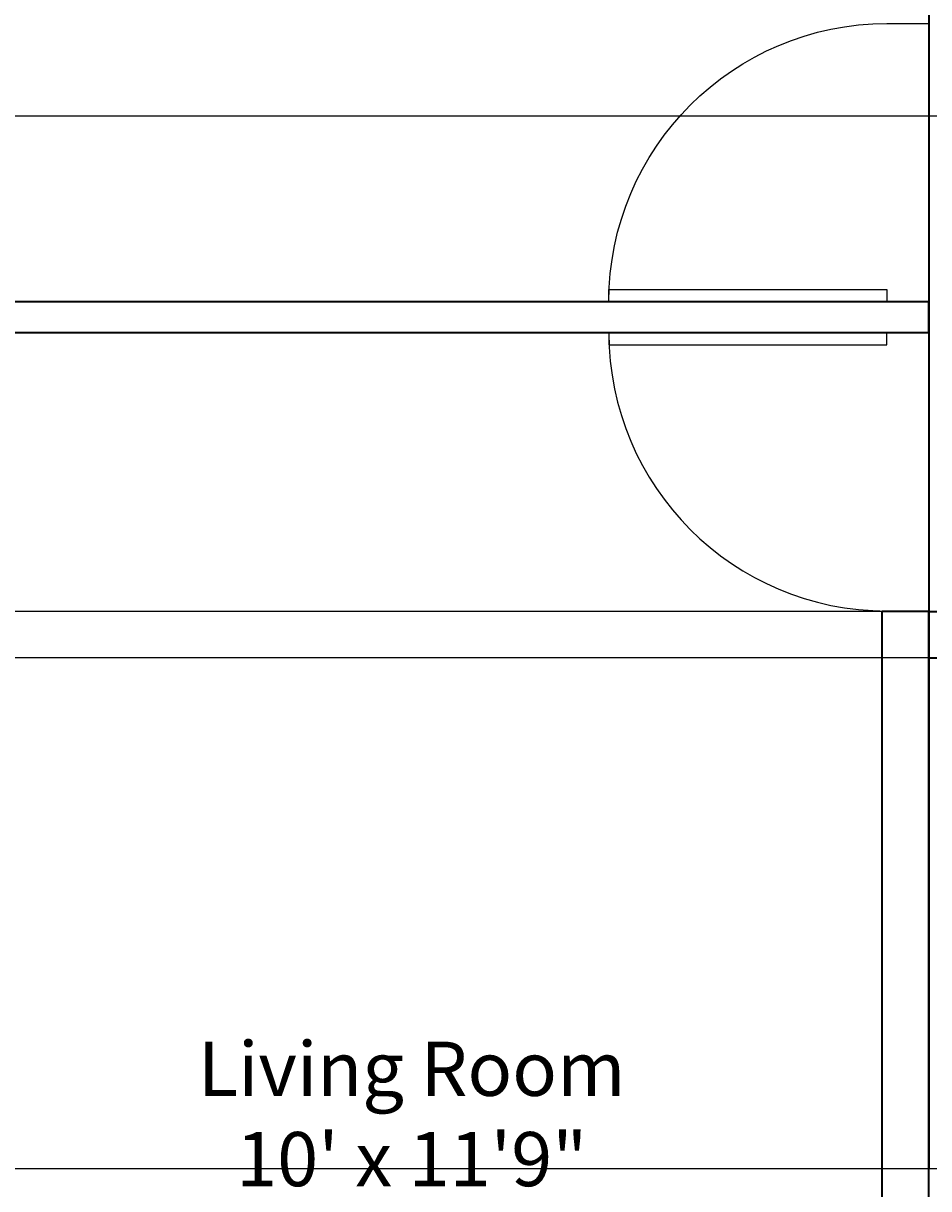
# Model space of a CAD drawing. Units: feet. Extents: x 105 to 1094, y -88 to 588.
# Tile 36 of 59: x 436 to 553, y 138 to 288. Entities that reach past the tile are written whole.
import ezdxf

# ---------------------------------------------------------------- set-up
doc = ezdxf.new("R2010")
doc.units = ezdxf.units.FT
doc.header["$MEASUREMENT"] = 0
for name, color, linetype, lineweight in [('A-ANNO-DIMS', 2, 'Continuous', 18), ('A-AREA-IDEN', 7, 'Continuous', 18), ('A-DOOR', 3, 'Continuous', 25), ('A-WALL', 7, 'Continuous', 35)]:
    doc.layers.add(name, color=color, linetype=linetype, lineweight=lineweight)
doc.styles.get("Standard").update_dxf_attribs({"font": 'arial.ttf'})
doc.dimstyles.get("Standard").update_dxf_attribs({"dimtxt": 0.18, "dimasz": 0.18, "dimexe": 0.18, "dimexo": 0.0625, "dimgap": 0.09, "dimtad": 0, "dimtih": 1, "dimtoh": 1, "dimdec": 4, "dimzin": 0, "dimdsep": 46, "dimtxsty": 'Standard', "dimcen": 0.09, "dimadec": 0, "dimazin": 0, "dimtfac": 1, "dimtdec": 4, "dimtofl": 0, "dimtmove": 0, "dimatfit": 3, "dimfxl": 1, "dimtolj": 1, "dimtzin": 0, "dimarcsym": 0})

# ---------------------------------------------------------------- blocks, each defined once
blk = doc.blocks.new('*U3')
for p, q in [((0, 0), (0, -6)), ((-40, 0), (-40, -6))]:
    blk.add_line(p, q)
blk.add_lwpolyline([(0, 0), (0, 40), (-1.75, 40), (-1.75, 0)], close=True)
blk.add_arc((0, 0), 40, 90, 180)
blk = doc.blocks.new('*D20')
at = {"layer": 'A-ANNO-DIMS', "color": 0, "lineweight": -2, "transparency": 16777216}
for p, q in [((150.69, 276.02), (150.69, -88.15)), ((1048.69, 276.02), (1048.69, -88.15)), ((150.87, -87.97), (599.4, -87.97)), ((1048.51, -87.97), (599.98, -87.97))]:
    blk.add_line(p, q, dxfattribs=at)
at = {"layer": 'A-ANNO-DIMS', "color": 0, "transparency": 16777216}
for points in [[(150.87, -87.94), (150.87, -88), (150.69, -87.97)], [(1048.51, -87.94), (1048.51, -88), (1048.69, -87.97)]]:
    blk.add_solid(points, dxfattribs=at)
at = {"layer": 'Defpoints', "color": 0, "transparency": 16777216}
for p in [(150.69, 276.08), (1048.69, 276.08), (1048.69, -87.97)]:
    blk.add_point(p, dxfattribs=at)
at = {"layer": 'A-ANNO-DIMS', "color": 0, "transparency": 16777216, "insert": (599.69, -87.97), "char_height": 0.18, "attachment_point": 5}
blk.add_mtext('\\A1;898', dxfattribs=at)
blk = doc.blocks.new('*D21')
at = {"layer": 'A-ANNO-DIMS', "color": 0, "lineweight": -2, "transparency": 16777216}
for p, q in [((849.63, 543.08), (105.46, 543.08)), ((105.64, 542.9), (105.64, 250.26)), ((105.64, -42.74), (105.64, 249.9)), ((849.63, -42.92), (105.46, -42.92))]:
    blk.add_line(p, q, dxfattribs=at)
at = {"layer": 'A-ANNO-DIMS', "color": 0, "transparency": 16777216}
for points in [[(105.61, 542.9), (105.67, 542.9), (105.64, 543.08)], [(105.61, -42.74), (105.67, -42.74), (105.64, -42.92)]]:
    blk.add_solid(points, dxfattribs=at)
at = {"layer": 'Defpoints', "color": 0, "transparency": 16777216}
for p in [(105.64, 543.08), (849.69, 543.08), (849.69, -42.92)]:
    blk.add_point(p, dxfattribs=at)
at = {"layer": 'A-ANNO-DIMS', "color": 0, "transparency": 16777216, "insert": (105.64, 250.08), "char_height": 0.18, "attachment_point": 5}
blk.add_mtext('\\A1;586', dxfattribs=at)
blk = doc.blocks.new('*D36')
at = {"layer": 'A-ANNO-DIMS', "color": 0, "lineweight": -2, "transparency": 16777216}
for p, q in [((547.24, 248.08), (105.46, 248.08)), ((105.64, 247.9), (105.64, 230.26)), ((105.64, 212.26), (105.64, 229.9)), ((546.63, 212.08), (105.46, 212.08))]:
    blk.add_line(p, q, dxfattribs=at)
at = {"layer": 'A-ANNO-DIMS', "color": 0, "transparency": 16777216}
for points in [[(105.61, 247.9), (105.67, 247.9), (105.64, 248.08)], [(105.61, 212.26), (105.67, 212.26), (105.64, 212.08)]]:
    blk.add_solid(points, dxfattribs=at)
at = {"layer": 'Defpoints', "color": 0, "transparency": 16777216}
for p in [(105.64, 248.08), (547.3, 248.08), (546.69, 212.08)]:
    blk.add_point(p, dxfattribs=at)
at = {"layer": 'A-ANNO-DIMS', "color": 0, "transparency": 16777216, "insert": (105.64, 230.08), "char_height": 0.18, "attachment_point": 5}
blk.add_mtext('\\A1;36', dxfattribs=at)
blk = doc.blocks.new('*D46')
at = {"layer": 'A-ANNO-DIMS', "color": 0, "lineweight": -2, "transparency": 16777216}
for p, q in [((580.63, 206.08), (105.46, 206.08)), ((105.64, 205.9), (105.64, 173.26)), ((105.64, 140.26), (105.64, 172.9)), ((580.63, 140.08), (105.46, 140.08))]:
    blk.add_line(p, q, dxfattribs=at)
at = {"layer": 'A-ANNO-DIMS', "color": 0, "transparency": 16777216}
for points in [[(105.61, 205.9), (105.67, 205.9), (105.64, 206.08)], [(105.61, 140.26), (105.67, 140.26), (105.64, 140.08)]]:
    blk.add_solid(points, dxfattribs=at)
at = {"layer": 'Defpoints', "color": 0, "transparency": 16777216}
for p in [(580.69, 206.08), (105.64, 140.08), (580.69, 140.08)]:
    blk.add_point(p, dxfattribs=at)
at = {"layer": 'A-ANNO-DIMS', "color": 0, "transparency": 16777216, "insert": (105.64, 173.08), "char_height": 0.18, "attachment_point": 5}
blk.add_mtext('\\A1;66', dxfattribs=at)
blk = doc.blocks.new('*D54')
at = {"layer": 'A-ANNO-DIMS', "color": 0, "lineweight": -2, "transparency": 16777216}
for p, q in [((294.75, 296.08), (1093.92, 296.08)), ((1093.74, 295.9), (1093.74, 286.26)), ((1093.74, 276.26), (1093.74, 285.9)), ((294.75, 276.08), (1093.92, 276.08))]:
    blk.add_line(p, q, dxfattribs=at)
at = {"layer": 'A-ANNO-DIMS', "color": 0, "transparency": 16777216}
for points in [[(1093.71, 295.9), (1093.77, 295.9), (1093.74, 296.08)], [(1093.71, 276.26), (1093.77, 276.26), (1093.74, 276.08)]]:
    blk.add_solid(points, dxfattribs=at)
at = {"layer": 'Defpoints', "color": 0, "transparency": 16777216}
for p in [(294.69, 296.08), (1093.74, 296.08), (294.69, 276.08)]:
    blk.add_point(p, dxfattribs=at)
at = {"layer": 'A-ANNO-DIMS', "color": 0, "transparency": 16777216, "insert": (1093.74, 286.08), "char_height": 0.18, "attachment_point": 5}
blk.add_mtext('\\A1;20', dxfattribs=at)

msp = doc.modelspace()

# ---------------------------------------------------------------- linework, layer by layer
at = {"layer": 'A-WALL'}
for p, q in [((552.6883, 295.0812), (552.6883, 206.0812)), ((552.6883, 252.0812), (370.6883, 252.0812)), ((552.6883, 252.0812), (426.6883, 252.0812)), ((552.6883, 252.0812), (552.6883, 248.0812)), ((552.6883, 248.0812), (552.6883, 252.0812)), ((552.6883, 248.0812), (370.6883, 248.0812)), ((552.6883, 248.0812), (426.6883, 248.0812)), ((552.6883, 248.0812), (552.6883, 140.0812)), ((552.6883, 212.0812), (546.6883, 212.0812)), ((546.6883, 65.0812), (546.6883, 212.0812)), ((552.6883, 212.0812), (646.6883, 212.0812)), ((552.6883, 59.0812), (552.6883, 212.0812)), ((552.6883, 206.0812), (580.6883, 206.0812))]:
    msp.add_line(p, q, dxfattribs=at)

# ---------------------------------------------------------------- block references
at = {"layer": 'A-DOOR', "yscale": 0.8984622266767051, "zscale": 0.8984622266767051}
for p, xscale, rotation in [((547.2975, 252.0812), -0.8984622266767051, 90), ((547.2975, 248.0812), 0.8984622266767051, 90.00000000000003)]:
    msp.add_blockref('*U3', p, dxfattribs=dict(at, xscale=xscale, rotation=rotation))

# ---------------------------------------------------------------- texts
at = {"layer": 'A-AREA-IDEN', "insert": (535.0519, 137.8526), "char_height": 7, "attachment_point": 9}
msp.add_mtext_dynamic_manual_height_columns('\\pxqc;Living Room \\P10\' x 11\'9"', width=98.34246, gutter_width=1, heights=[0], dxfattribs=at)

# ---------------------------------------------------------------- dimensions: what is measured, and where the dimension line sits
at = {"layer": 'A-ANNO-DIMS'}
for base, p1, p2, picture, middle in [((105.6383, 543.0812), (849.6883, -42.9188), (849.6883, 543.0812), '*D21', (105.6383, 250.0812)), ((1093.7383, 296.0812), (294.6883, 276.0812), (294.6883, 296.0812), '*D54', (1093.7383, 286.0812)), ((105.6383, 248.0812), (546.6883, 212.0812), (547.2975, 248.0812), '*D36', (105.6383, 230.0812)), ((105.6383, 140.0812), (580.6883, 206.0812), (580.6883, 140.0812), '*D46', (105.6383, 173.0812))]:
    dim = msp.add_linear_dim(base=base, p1=p1, p2=p2, angle=90, dimstyle='Standard', override={"dimdec": 0, "dimlfac": 1, "dimrnd": 0, "dimzin": 0, "dimdsep": 46, "dimlunit": 2}, dxfattribs=at)
    dim.commit()
    dim.dimension.update_dxf_attribs({"geometry": picture, "text_midpoint": middle})
dim = msp.add_linear_dim(base=(1048.6883, -87.9688), p1=(150.6883, 276.0812), p2=(1048.6883, 276.0812), dimstyle='Standard', override={"dimdec": 0, "dimlfac": 1, "dimrnd": 0, "dimzin": 0, "dimdsep": 46, "dimlunit": 2}, dxfattribs=at)
dim.commit()
dim.dimension.update_dxf_attribs({"geometry": '*D20', "text_midpoint": (599.6883, -87.9688)})

doc.saveas('drawing.dxf')
